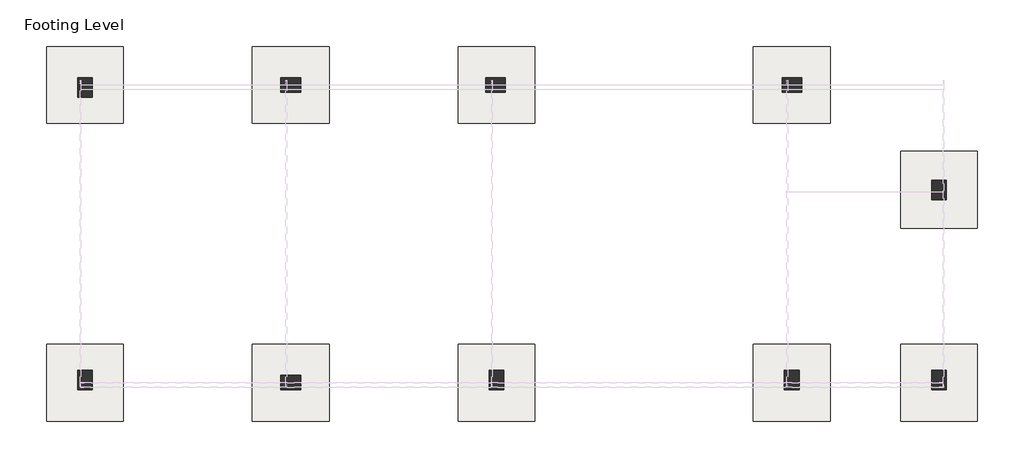
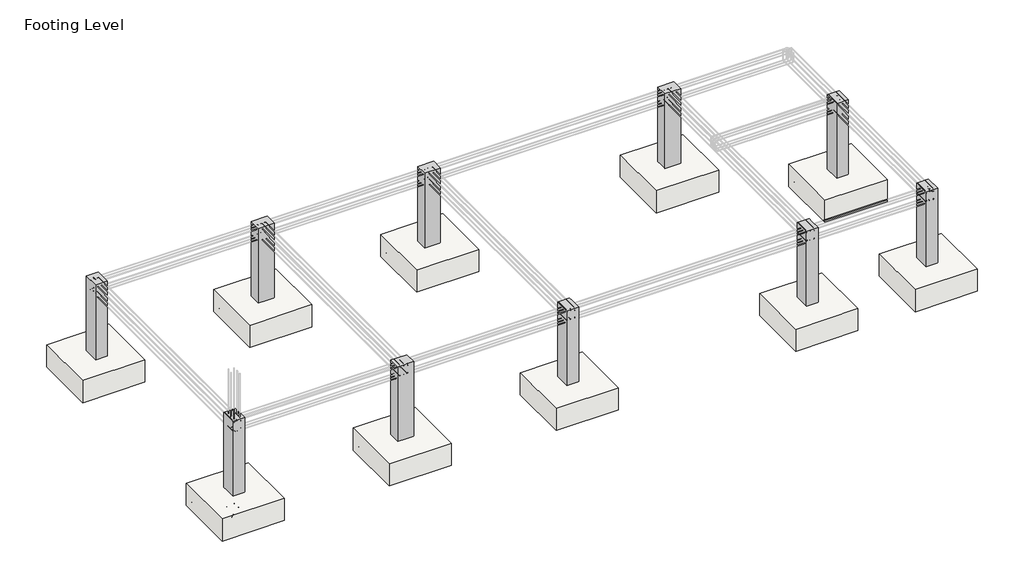
# One storey, part 1 of 3: 10 columns, 10 slabs.
"""IFC4 building model written with IfcOpenShell, lengths in millimetres."""

from ifc_helpers import new_model, si_unit, frame, origin, place, context, project, spatial, polyline, outline, extrude, faceted_brep, transform, mapped, element, save
from components import m_footing_rectangular_1200_x1200_x450_1789818b

model = new_model("IFC4")

# Units and contexts
model_context = context("Model", 3, world=origin())
ifc_project = project(units=[si_unit("LENGTHUNIT", "METRE", prefix="MILLI")], contexts=[model_context])

# Site, building, storey
site = spatial("IfcSite", under=ifc_project)
building = spatial("IfcBuilding", under=site)
storey = spatial("IfcBuildingStorey", under=building, Name="Footing Level", Elevation=-1524.0)

# Columns
placement = place(None, origin())
element("IfcColumn", 1, ObjectType="M_Concrete-Rectangular-Column : 9\" x 12\"", at=placement, inside=storey, context=model_context, shape_type="SweptSolid", body=[
    extrude(outline(polyline([(-9150.3117524, 5063.2334631), (-9150.3117524, 4758.4334631), (-9378.9117524, 4758.4334631), (-9378.9117524, 5063.2334631), (-9150.3117524, 5063.2334631)])), frame((0.0, 0.0, -1524.0), z_axis=(0.0, 0.0, 1.0), x_axis=(1.0, 0.0, 0.0)), (0.0, 0.0, 1.0), 1524.0),
])
element("IfcColumn", 2, ObjectType="M_Concrete-Rectangular-Column : 9\" x 12\"", at=placement, inside=storey, context=model_context, shape_type="SweptSolid", body=[
    extrude(outline(polyline([(-9150.3117524, 491.2334631), (-9150.3117524, 186.4334631), (-9378.9117524, 186.4334631), (-9378.9117524, 491.2334631), (-9150.3117524, 491.2334631)])), frame((0.0, 0.0, -1524.0), z_axis=(0.0, 0.0, 1.0), x_axis=(1.0, 0.0, 0.0)), (0.0, 0.0, 1.0), 1524.0),
])
element("IfcColumn", 3, ObjectType="M_Concrete-Rectangular-Column : 9\" x 12\"", at=placement, inside=storey, context=model_context, shape_type="Brep", body=[
    faceted_brep([(-6203.9117524, 415.0334631, -1524.0), (-5899.1117524, 415.0334631, -1524.0), (-5899.1117524, 186.4334631, -1524.0), (-6203.9117524, 186.4334631, -1524.0), (-6203.9117524, 415.0334631, 0.0), (-5899.1117524, 415.0334631, 0.0), (-5899.1117524, 415.0334631, -304.8), (-6203.9117524, 415.0334631, -304.8), (-5899.1117524, 186.4334631, 0.0), (-5899.1117524, 186.4334631, -304.8), (-6203.9117524, 186.4334631, 0.0), (-6203.9117524, 186.4334631, -304.8)], [[[0, 1, 2, 3]], [[4, 5, 6, 1, 0, 7]], [[5, 8, 9, 2, 1, 6]], [[8, 10, 11, 3, 2, 9]], [[10, 4, 7, 0, 3, 11]], [[4, 10, 8, 5]]]),
])
element("IfcColumn", 4, ObjectType="M_Concrete-Rectangular-Column : 9\" x 12\"", at=placement, inside=storey, context=model_context, shape_type="Brep", body=[
    faceted_brep([(-2952.7117524, 186.4334631, -1524.0), (-2952.7117524, 491.2334631, -1524.0), (-2724.1117524, 491.2334631, -1524.0), (-2724.1117524, 186.4334631, -1524.0), (-2952.7117524, 186.4334631, 0.0), (-2952.7117524, 415.0334631, 0.0), (-2952.7117524, 491.2334631, 0.0), (-2952.7117524, 186.4334631, -304.8), (-2724.1117524, 491.2334631, 0.0), (-2724.1117524, 415.0334631, 0.0), (-2724.1117524, 186.4334631, 0.0), (-2724.1117524, 186.4334631, -304.8)], [[[0, 1, 2, 3]], [[4, 5, 6, 1, 0, 7]], [[6, 8, 2, 1]], [[8, 9, 10, 11, 3, 2]], [[10, 4, 7, 0, 3, 11]], [[4, 10, 9, 8, 6, 5]]]),
])
element("IfcColumn", 5, ObjectType="M_Concrete-Rectangular-Column : 9\" x 12\"", at=placement, inside=storey, context=model_context, shape_type="Brep", body=[
    faceted_brep([(1657.3882476, 186.4334631, -1524.0), (1657.3882476, 491.2334631, -1524.0), (1885.9882476, 491.2334631, -1524.0), (1885.9882476, 186.4334631, -1524.0), (1657.3882476, 186.4334631, 0.0), (1657.3882476, 415.0334631, 0.0), (1657.3882476, 491.2334631, 0.0), (1657.3882476, 186.4334631, -304.8), (1885.9882476, 491.2334631, 0.0), (1885.9882476, 415.0334631, 0.0), (1885.9882476, 186.4334631, 0.0), (1885.9882476, 186.4334631, -304.8)], [[[0, 1, 2, 3]], [[4, 5, 6, 1, 0, 7]], [[6, 8, 2, 1]], [[8, 9, 10, 11, 3, 2]], [[10, 4, 7, 0, 3, 11]], [[4, 10, 9, 8, 6, 5]]]),
])
element("IfcColumn", 6, ObjectType="M_Concrete-Rectangular-Column : 9\" x 12\"", at=placement, inside=storey, context=model_context, shape_type="SweptSolid", body=[
    extrude(outline(polyline([(3956.0882476, 186.4334631), (3956.0882476, 491.2334631), (4184.6882476, 491.2334631), (4184.6882476, 186.4334631), (3956.0882476, 186.4334631)])), frame((0.0, 0.0, -1524.0), z_axis=(0.0, 0.0, 1.0), x_axis=(1.0, 0.0, 0.0)), (0.0, 0.0, 1.0), 1524.0),
])
element("IfcColumn", 7, ObjectType="M_Concrete-Rectangular-Column : 9\" x 12\"", at=placement, inside=storey, context=model_context, shape_type="Brep", body=[
    faceted_brep([(3956.0882476, 3158.2334631, -1524.0), (3956.0882476, 3463.0334631, -1524.0), (4184.6882476, 3463.0334631, -1524.0), (4184.6882476, 3158.2334631, -1524.0), (3956.0882476, 3158.2334631, 0.0), (3956.0882476, 3463.0334631, 0.0), (3956.0882476, 3463.0334631, -304.8), (3956.0882476, 3158.2334631, -304.8), (4184.6882476, 3463.0334631, 0.0), (4184.6882476, 3463.0334631, -304.8), (4184.6882476, 3158.2334631, 0.0), (4184.6882476, 3158.2334631, -304.8)], [[[0, 1, 2, 3]], [[4, 5, 6, 1, 0, 7]], [[5, 8, 9, 2, 1, 6]], [[8, 10, 11, 3, 2, 9]], [[10, 4, 7, 0, 3, 11]], [[4, 10, 8, 5]]]),
])
element("IfcColumn", 8, ObjectType="M_Concrete-Rectangular-Column : 9\" x 12\"", at=placement, inside=storey, context=model_context, shape_type="Brep", body=[
    faceted_brep([(1924.0882476, 4834.6334631, -1524.0), (1619.2882476, 4834.6334631, -1524.0), (1619.2882476, 5063.2334631, -1524.0), (1924.0882476, 5063.2334631, -1524.0), (1924.0882476, 4834.6334631, 0.0), (1619.2882476, 4834.6334631, 0.0), (1619.2882476, 4834.6334631, -304.8), (1924.0882476, 4834.6334631, -304.8), (1619.2882476, 5063.2334631, 0.0), (1619.2882476, 5063.2334631, -304.8), (1924.0882476, 5063.2334631, 0.0), (1924.0882476, 5063.2334631, -304.8)], [[[0, 1, 2, 3]], [[4, 5, 6, 1, 0, 7]], [[5, 8, 9, 2, 1, 6]], [[8, 10, 11, 3, 2, 9]], [[10, 4, 7, 0, 3, 11]], [[4, 10, 8, 5]]]),
])
element("IfcColumn", 9, ObjectType="M_Concrete-Rectangular-Column : 9\" x 12\"", at=placement, inside=storey, context=model_context, shape_type="Brep", body=[
    faceted_brep([(-2698.7117524, 4834.6334631, -1524.0), (-3003.5117524, 4834.6334631, -1524.0), (-3003.5117524, 5063.2334631, -1524.0), (-2698.7117524, 5063.2334631, -1524.0), (-2698.7117524, 4834.6334631, 0.0), (-3003.5117524, 4834.6334631, 0.0), (-3003.5117524, 4834.6334631, -304.8), (-2698.7117524, 4834.6334631, -304.8), (-3003.5117524, 5063.2334631, 0.0), (-3003.5117524, 5063.2334631, -304.8), (-2698.7117524, 5063.2334631, 0.0), (-2698.7117524, 5063.2334631, -304.8)], [[[0, 1, 2, 3]], [[4, 5, 6, 1, 0, 7]], [[5, 8, 9, 2, 1, 6]], [[8, 10, 11, 3, 2, 9]], [[10, 4, 7, 0, 3, 11]], [[4, 10, 8, 5]]]),
])
element("IfcColumn", 10, ObjectType="M_Concrete-Rectangular-Column : 9\" x 12\"", at=placement, inside=storey, context=model_context, shape_type="Brep", body=[
    faceted_brep([(-5899.1117524, 4834.6334631, -1524.0), (-6203.9117524, 4834.6334631, -1524.0), (-6203.9117524, 5063.2334631, -1524.0), (-5899.1117524, 5063.2334631, -1524.0), (-5899.1117524, 4834.6334631, 0.0), (-6203.9117524, 4834.6334631, 0.0), (-6203.9117524, 4834.6334631, -304.8), (-5899.1117524, 4834.6334631, -304.8), (-6203.9117524, 5063.2334631, 0.0), (-6203.9117524, 5063.2334631, -304.8), (-5899.1117524, 5063.2334631, 0.0), (-5899.1117524, 5063.2334631, -304.8)], [[[0, 1, 2, 3]], [[4, 5, 6, 1, 0, 7]], [[5, 8, 9, 2, 1, 6]], [[8, 10, 11, 3, 2, 9]], [[10, 4, 7, 0, 3, 11]], [[4, 10, 8, 5]]]),
])

# Slabs
m_footing_rectangular_1200_x1200_x450_shape = m_footing_rectangular_1200_x1200_x450_1789818b(model_context)
element("IfcSlab", 11, ObjectType="M_Footing-Rectangular : 1200 X1200 X450", at=placement, inside=storey, context=model_context, shape_type="MappedRepresentation", body=[
    mapped(m_footing_rectangular_1200_x1200_x450_shape, transform((-9264.6117524, 300.7334631, -1524.0), x_axis=(1.0, 0.0, 0.0), y_axis=(0.0, 1.0, 0.0), z_axis=(0.0, 0.0, 1.0))),
])
element("IfcSlab", 12, ObjectType="M_Footing-Rectangular : 1200 X1200 X450", at=placement, inside=storey, context=model_context, shape_type="MappedRepresentation", body=[
    mapped(m_footing_rectangular_1200_x1200_x450_shape, transform((-9264.6117524, 4948.9334631, -1524.0), x_axis=(1.0, 0.0, 0.0), y_axis=(0.0, 1.0, 0.0), z_axis=(0.0, 0.0, 1.0))),
])
element("IfcSlab", 13, ObjectType="M_Footing-Rectangular : 1200 X1200 X450", at=placement, inside=storey, context=model_context, shape_type="MappedRepresentation", body=[
    mapped(m_footing_rectangular_1200_x1200_x450_shape, transform((-6051.5117524, 300.7334631, -1524.0), x_axis=(1.0, 0.0, 0.0), y_axis=(0.0, 1.0, 0.0), z_axis=(0.0, 0.0, 1.0))),
])
element("IfcSlab", 14, ObjectType="M_Footing-Rectangular : 1200 X1200 X450", at=placement, inside=storey, context=model_context, shape_type="MappedRepresentation", body=[
    mapped(m_footing_rectangular_1200_x1200_x450_shape, transform((-6051.5117524, 4948.9334631, -1524.0), x_axis=(1.0, 0.0, 0.0), y_axis=(0.0, 1.0, 0.0), z_axis=(0.0, 0.0, 1.0))),
])
element("IfcSlab", 15, ObjectType="M_Footing-Rectangular : 1200 X1200 X450", at=placement, inside=storey, context=model_context, shape_type="MappedRepresentation", body=[
    mapped(m_footing_rectangular_1200_x1200_x450_shape, transform((-2838.4117524, 300.7334631, -1524.0), x_axis=(1.0, 0.0, 0.0), y_axis=(0.0, 1.0, 0.0), z_axis=(0.0, 0.0, 1.0))),
])
element("IfcSlab", 16, ObjectType="M_Footing-Rectangular : 1200 X1200 X450", at=placement, inside=storey, context=model_context, shape_type="MappedRepresentation", body=[
    mapped(m_footing_rectangular_1200_x1200_x450_shape, transform((-2838.4117524, 4948.9334631, -1524.0), x_axis=(1.0, 0.0, 0.0), y_axis=(0.0, 1.0, 0.0), z_axis=(0.0, 0.0, 1.0))),
])
element("IfcSlab", 17, ObjectType="M_Footing-Rectangular : 1200 X1200 X450", at=placement, inside=storey, context=model_context, shape_type="MappedRepresentation", body=[
    mapped(m_footing_rectangular_1200_x1200_x450_shape, transform((1771.6882476, 300.7334631, -1524.0), x_axis=(1.0, 0.0, 0.0), y_axis=(0.0, 1.0, 0.0), z_axis=(0.0, 0.0, 1.0))),
])
element("IfcSlab", 18, ObjectType="M_Footing-Rectangular : 1200 X1200 X450", at=placement, inside=storey, context=model_context, shape_type="MappedRepresentation", body=[
    mapped(m_footing_rectangular_1200_x1200_x450_shape, transform((1771.6882476, 4948.9334631, -1524.0), x_axis=(1.0, 0.0, 0.0), y_axis=(0.0, 1.0, 0.0), z_axis=(0.0, 0.0, 1.0))),
])
element("IfcSlab", 19, ObjectType="M_Footing-Rectangular : 1200 X1200 X450", at=placement, inside=storey, context=model_context, shape_type="MappedRepresentation", body=[
    mapped(m_footing_rectangular_1200_x1200_x450_shape, transform((4070.3882476, 300.7334631, -1524.0), x_axis=(1.0, 0.0, 0.0), y_axis=(0.0, 1.0, 0.0), z_axis=(0.0, 0.0, 1.0))),
])
element("IfcSlab", 20, ObjectType="M_Footing-Rectangular : 1200 X1200 X450", at=placement, inside=storey, context=model_context, shape_type="MappedRepresentation", body=[
    mapped(m_footing_rectangular_1200_x1200_x450_shape, transform((4070.3882476, 3310.6334631, -1524.0), x_axis=(1.0, 0.0, 0.0), y_axis=(0.0, 1.0, 0.0), z_axis=(0.0, 0.0, 1.0))),
])

save(model, "model.ifc")

# Revit data of these elements
# Grids (mm)
#   "1": line (-9264.612, 7188.168) -> (-9264.612, -912.383)
#   "2": line (-6051.512, 7188.168) -> (-6051.512, -912.383)
#   "3": line (-2838.412, 7188.168) -> (-2838.412, -912.383)
#   "4": line (1771.688, 7188.168) -> (1771.688, -912.383)
#   "5": line (4070.388, 7188.168) -> (4070.388, -912.383)
#   "A": line (8119.701, 300.733) -> (-11364.612, 300.733)
#   "B": line (8199.349, 4948.933) -> (-11364.612, 4948.933)
# Type "M_Concrete-Rectangular-Column : 9\" x 12\""
#   b = 0' - 9"
#   h = 1' - 0"
#   Structural Material [instance default] = Concrete, Cast-in-Place gray
# Type "M_Footing-Rectangular : 1200 X1200 X450"
#   Width = 3' - 11.24409"
#   Length = 3' - 11.24409"
#   Foundation Thickness = 1' - 5.71654"
#   Structural Material [instance default] = Concrete, Cast-in-Place gray
#   Assembly Code = ""
# Elements 1, 2, 3, 4, 5, 6, 7, 8, 9, 10 (IfcColumn, "M_Concrete-Rectangular-Column : 9\" x 12\"")
#   Structural Material = Concrete, Cast-in-Place gray
#   Phase Created = New Construction
#   Materials on its faces: "Concrete, Cast-in-Place gray"
# Elements 11, 12, 13, 14, 15, 16, 17, 18, 19, 20 (IfcSlab, "M_Footing-Rectangular : 1200 X1200 X450")
#   Structural Material = Concrete, Cast-in-Place gray
#   Phase Created = New Construction
#   Materials on its faces: "Concrete, Cast-in-Place gray"
# Materials
#   "Concrete, Cast-in-Place gray": class "Concrete", colour RGB 192 192 192, transparency 0, Description = "Cast-in-place concrete", Cost = 0
